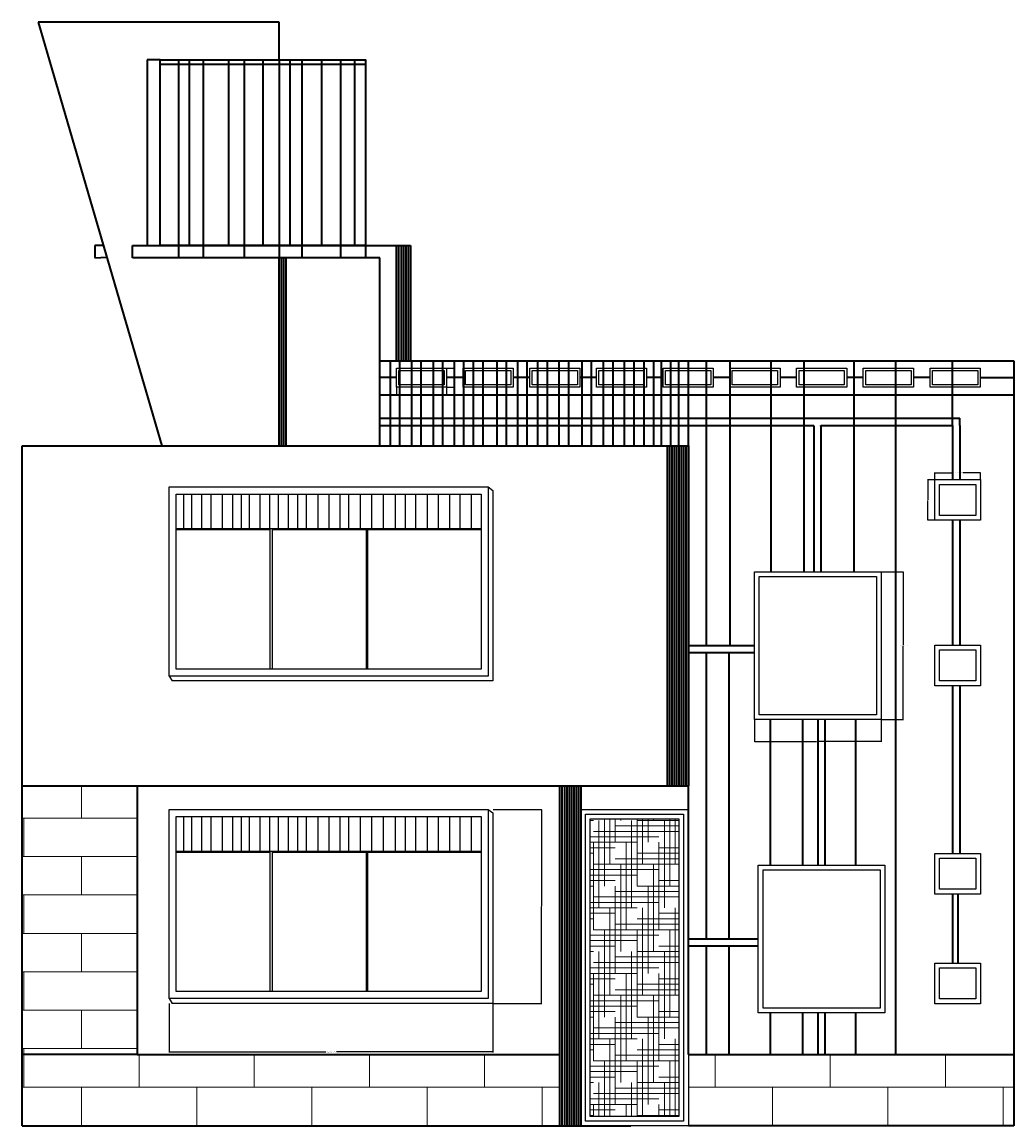
# Model space of a CAD drawing. Units: inches. Extents: x 72 to 493, y 65 to 532.
import ezdxf

# ---------------------------------------------------------------- set-up
doc = ezdxf.new("R2010")
doc.units = ezdxf.units.IN
doc.header["$MEASUREMENT"] = 0
for name, color, linetype, lineweight in [('A-ANNO-DIMS', 2, 'Continuous', 18), ('A-DOOR', 3, 'Continuous', 25), ('A-DOOR-PATT', 8, 'Continuous', 13), ('A-ELEV', 7, 'Continuous', 35), ('A-GLAZ', 4, 'Continuous', 25), ('A-WALL-PATT', 8, 'Continuous', 13)]:
    doc.layers.add(name, color=color, linetype=linetype, lineweight=lineweight)
doc.styles.get("Standard").update_dxf_attribs({"font": 'arial.ttf'})
doc.dimstyles.get("Standard").update_dxf_attribs({"dimtxt": 0.18, "dimasz": 0.18, "dimexe": 0.18, "dimexo": 0.0625, "dimgap": 0.09, "dimtad": 0, "dimtih": 1, "dimtoh": 1, "dimdec": 4, "dimzin": 0, "dimdsep": 46, "dimtxsty": 'Standard', "dimcen": 0.09, "dimadec": 0, "dimazin": 0, "dimtfac": 1, "dimtdec": 4, "dimtofl": 0, "dimtmove": 0, "dimatfit": 3, "dimfxl": 1, "dimtolj": 1, "dimtzin": 0, "dimarcsym": 0})

# ---------------------------------------------------------------- blocks, each defined once
blk = doc.blocks.new('WIN-SLIDING-3P')
for p, q in [((135.19, 82.11), (137.19, 80.63)), ((6.15, 79.11), (6.15, 64.5)), ((9.47, 79.11), (9.47, 64.5)), ((13.66, 79.11), (13.66, 64.5)), ((17.62, 79.11), (17.62, 64.5)), ((22.45, 79.11), (22.45, 64.5)), ((26.79, 79.11), (26.79, 64.5)), ((30.5, 79.11), (30.5, 64.5)), ((33.96, 79.11), (33.96, 64.5)), ((38.45, 79.11), (38.45, 64.5)), ((42.5, 79.11), (42.5, 64.5)), ((46.21, 79.11), (46.21, 64.5)), ((50.45, 79.11), (50.45, 64.5)), ((54.35, 79.11), (54.35, 64.5)), ((58.03, 79.11), (58.03, 64.5)), ((62.95, 79.11), (62.95, 64.5)), ((67.59, 79.11), (67.59, 64.5)), ((72.27, 79.11), (72.27, 64.5)), ((75.98, 79.11), (75.98, 64.5)), ((80.86, 79.11), (80.86, 64.5)), ((85.7, 79.11), (85.7, 64.5)), ((90.63, 79.11), (90.63, 64.5)), ((95.8, 79.11), (95.8, 64.5)), ((100.04, 79.11), (100.04, 64.5)), ((104.4, 79.11), (104.4, 64.5)), ((109.37, 79.11), (109.37, 64.5)), ((113.96, 79.11), (113.96, 64.5)), ((118.79, 79.11), (118.79, 64.5)), ((123.13, 79.11), (123.13, 64.5)), ((128.01, 79.11), (128.01, 64.5)), ((3, 64.5), (132.19, 64.5)), ((0, 2), (1.28, 0))]:
    blk.add_line(p, q)
for points in [[(0, 82.11), (135.19, 82.11), (135.19, 2), (0, 2)], [(3, 79.11), (132.19, 79.11), (132.19, 5), (3, 5)], [(3, 64.05), (42.69, 64.05), (42.69, 5), (3, 5)], [(43.75, 64.05), (83.44, 64.05), (83.44, 5), (43.75, 5)], [(84.24, 64.05), (132.19, 64.05), (132.19, 5), (84.24, 5)]]:
    blk.add_lwpolyline(points, close=True)
blk.add_lwpolyline([(137.19, 80.63), (137.19, 0), (1.28, 0)])
blk = doc.blocks.new('WIN-CLERESTORY')
for points in [[(0, 8.05), (21.2, 8.05), (21.2, 0), (0, 0)], [(1, 7.05), (20.2, 7.05), (20.2, 1), (1, 1)]]:
    blk.add_lwpolyline(points, close=True)
blk = doc.blocks.new('WIN-SQ-SMALL')
for points in [[(0, 17.16), (19.41, 17.16), (19.41, 0), (0, 0)], [(2, 15.16), (17.41, 15.16), (17.41, 2), (2, 2)]]:
    blk.add_lwpolyline(points, close=True)
blk = doc.blocks.new('WIN-SQ-LARGE')
for points in [[(0, 62.56), (53.66, 62.56), (53.66, 0), (0, 0)], [(2, 60.56), (51.66, 60.56), (51.66, 2), (2, 2)]]:
    blk.add_lwpolyline(points, close=True)
blk = doc.blocks.new('*D5')
at = {"layer": 'A-ANNO-DIMS', "color": 0, "lineweight": -2, "transparency": 16777216}
for p, q in [((231.1, 377.71), (231.1, 374.41)), ((231.28, 374.59), (239.7, 374.59)), ((252.13, 374.59), (243.7, 374.59)), ((252.31, 377.71), (252.31, 374.41))]:
    blk.add_line(p, q, dxfattribs=at)
at = {"layer": 'A-ANNO-DIMS', "color": 0, "transparency": 16777216}
for points in [[(231.28, 374.62), (231.28, 374.56), (231.1, 374.59)], [(252.13, 374.62), (252.13, 374.56), (252.31, 374.59)]]:
    blk.add_solid(points, dxfattribs=at)
at = {"layer": 'Defpoints', "color": 0, "transparency": 16777216}
for p in [(231.1, 377.77), (252.31, 377.77), (252.31, 374.59)]:
    blk.add_point(p, dxfattribs=at)
at = {"layer": 'A-ANNO-DIMS', "color": 0, "transparency": 16777216, "insert": (241.7, 374.59), "char_height": 0.18, "attachment_point": 5}
blk.add_mtext('\\A1;CLERESTORY WINDOW 21 TYP.', dxfattribs=at)
blk = doc.blocks.new('*D6')
at = {"layer": 'A-ANNO-DIMS', "color": 0, "lineweight": -2, "transparency": 16777216}
for p, q in [((252.37, 385.83), (255.67, 385.83)), ((255.49, 385.65), (255.49, 381.98)), ((255.49, 377.95), (255.49, 381.62)), ((252.37, 377.77), (255.67, 377.77))]:
    blk.add_line(p, q, dxfattribs=at)
at = {"layer": 'A-ANNO-DIMS', "color": 0, "transparency": 16777216}
for points in [[(255.46, 385.65), (255.52, 385.65), (255.49, 385.83)], [(255.46, 377.95), (255.52, 377.95), (255.49, 377.77)]]:
    blk.add_solid(points, dxfattribs=at)
at = {"layer": 'Defpoints', "color": 0, "transparency": 16777216}
for p in [(252.31, 385.83), (255.49, 385.83), (252.31, 377.77)]:
    blk.add_point(p, dxfattribs=at)
at = {"layer": 'A-ANNO-DIMS', "color": 0, "transparency": 16777216, "insert": (255.49, 381.8), "char_height": 0.18, "attachment_point": 5}
blk.add_mtext('\\A1;8 TYP.', dxfattribs=at)
blk = doc.blocks.new('*D7')
at = {"layer": 'A-ANNO-DIMS', "color": 0, "lineweight": -2, "transparency": 16777216}
for p, q in [((459.13, 338.66), (459.13, 341.69)), ((459.31, 341.51), (466.71, 341.51)), ((478.36, 341.51), (470.96, 341.51)), ((478.54, 338.66), (478.54, 341.69))]:
    blk.add_line(p, q, dxfattribs=at)
at = {"layer": 'A-ANNO-DIMS', "color": 0, "transparency": 16777216}
for points in [[(459.31, 341.54), (459.31, 341.48), (459.13, 341.51)], [(478.36, 341.54), (478.36, 341.48), (478.54, 341.51)]]:
    blk.add_solid(points, dxfattribs=at)
at = {"layer": 'Defpoints', "color": 0, "transparency": 16777216}
for p in [(478.54, 341.51), (459.13, 338.59), (478.54, 338.59)]:
    blk.add_point(p, dxfattribs=at)
at = {"layer": 'A-ANNO-DIMS', "color": 0, "transparency": 16777216, "insert": (468.84, 341.51), "char_height": 0.18, "attachment_point": 5}
blk.add_mtext('\\A1;SMALL SQUARE WINDOW 19 TYP.', dxfattribs=at)
blk = doc.blocks.new('*D8')
at = {"layer": 'A-ANNO-DIMS', "color": 0, "lineweight": -2, "transparency": 16777216}
for p, q in [((459.07, 338.59), (456.04, 338.59)), ((456.22, 338.41), (456.22, 330.2)), ((456.22, 321.62), (456.22, 329.83)), ((459.07, 321.44), (456.04, 321.44))]:
    blk.add_line(p, q, dxfattribs=at)
at = {"layer": 'A-ANNO-DIMS', "color": 0, "transparency": 16777216}
for points in [[(456.19, 338.41), (456.25, 338.41), (456.22, 338.59)], [(456.19, 321.62), (456.25, 321.62), (456.22, 321.44)]]:
    blk.add_solid(points, dxfattribs=at)
at = {"layer": 'Defpoints', "color": 0, "transparency": 16777216}
for p in [(456.22, 338.59), (459.13, 338.59), (459.13, 321.44)]:
    blk.add_point(p, dxfattribs=at)
at = {"layer": 'A-ANNO-DIMS', "color": 0, "transparency": 16777216, "insert": (456.22, 330.02), "char_height": 0.18, "attachment_point": 5}
blk.add_mtext('\\A1;17 TYP.', dxfattribs=at)
blk = doc.blocks.new('*D9')
at = {"layer": 'A-ANNO-DIMS', "color": 0, "lineweight": -2, "transparency": 16777216}
for p, q in [((134.75, 116.73), (134.75, 96.04)), ((271.94, 116.73), (271.94, 96.04)), ((134.93, 96.22), (201.07, 96.22)), ((271.76, 96.22), (205.63, 96.22))]:
    blk.add_line(p, q, dxfattribs=at)
at = {"layer": 'A-ANNO-DIMS', "color": 0, "transparency": 16777216}
for points in [[(134.93, 96.25), (134.93, 96.19), (134.75, 96.22)], [(271.76, 96.25), (271.76, 96.19), (271.94, 96.22)]]:
    blk.add_solid(points, dxfattribs=at)
at = {"layer": 'Defpoints', "color": 0, "transparency": 16777216}
for p in [(134.75, 116.8), (271.94, 116.8), (271.94, 96.22)]:
    blk.add_point(p, dxfattribs=at)
at = {"layer": 'A-ANNO-DIMS', "color": 0, "transparency": 16777216, "insert": (203.35, 96.22), "char_height": 0.18, "attachment_point": 5}
blk.add_mtext('\\A1;3-PANEL SLIDING WINDOW 137 TYP.', dxfattribs=at)
blk = doc.blocks.new('*D10')
at = {"layer": 'A-ANNO-DIMS', "color": 0, "lineweight": -2, "transparency": 16777216}
for p, q in [((272, 198.91), (292.7, 198.91)), ((292.52, 198.73), (292.52, 158.03)), ((292.52, 116.98), (292.52, 157.67)), ((272, 116.8), (292.7, 116.8))]:
    blk.add_line(p, q, dxfattribs=at)
at = {"layer": 'A-ANNO-DIMS', "color": 0, "transparency": 16777216}
for points in [[(292.49, 198.73), (292.55, 198.73), (292.52, 198.91)], [(292.49, 116.98), (292.55, 116.98), (292.52, 116.8)]]:
    blk.add_solid(points, dxfattribs=at)
at = {"layer": 'Defpoints', "color": 0, "transparency": 16777216}
for p in [(271.94, 198.91), (292.52, 198.91), (271.94, 116.8)]:
    blk.add_point(p, dxfattribs=at)
at = {"layer": 'A-ANNO-DIMS', "color": 0, "transparency": 16777216, "insert": (292.52, 157.85), "char_height": 0.18, "attachment_point": 5}
blk.add_mtext('\\A1;82 TYP.', dxfattribs=at)
blk = doc.blocks.new('*D11')
at = {"layer": 'A-ANNO-DIMS', "color": 0, "lineweight": -2, "transparency": 16777216}
for p, q in [((436.42, 299.62), (445.92, 299.62)), ((445.74, 299.44), (445.74, 268.53)), ((445.74, 237.24), (445.74, 268.15)), ((436.42, 237.06), (445.92, 237.06))]:
    blk.add_line(p, q, dxfattribs=at)
at = {"layer": 'A-ANNO-DIMS', "color": 0, "transparency": 16777216}
for points in [[(445.71, 299.44), (445.77, 299.44), (445.74, 299.62)], [(445.71, 237.24), (445.77, 237.24), (445.74, 237.06)]]:
    blk.add_solid(points, dxfattribs=at)
at = {"layer": 'Defpoints', "color": 0, "transparency": 16777216}
for p in [(436.35, 299.62), (445.74, 299.62), (436.35, 237.06)]:
    blk.add_point(p, dxfattribs=at)
at = {"layer": 'A-ANNO-DIMS', "color": 0, "transparency": 16777216, "insert": (445.74, 268.34), "char_height": 0.18, "attachment_point": 5}
blk.add_mtext('\\A1;LARGE SQUARE WINDOW 63 TYP.', dxfattribs=at)
blk = doc.blocks.new('*D12')
at = {"layer": 'A-ANNO-DIMS', "color": 0, "lineweight": -2, "transparency": 16777216}
for p, q in [((382.7, 237), (382.7, 227.5)), ((436.35, 237), (436.35, 227.5)), ((382.88, 227.68), (409, 227.68)), ((436.17, 227.68), (410.05, 227.68))]:
    blk.add_line(p, q, dxfattribs=at)
at = {"layer": 'A-ANNO-DIMS', "color": 0, "transparency": 16777216}
for points in [[(382.88, 227.71), (382.88, 227.65), (382.7, 227.68)], [(436.17, 227.71), (436.17, 227.65), (436.35, 227.68)]]:
    blk.add_solid(points, dxfattribs=at)
at = {"layer": 'Defpoints', "color": 0, "transparency": 16777216}
for p in [(382.7, 237.06), (436.35, 237.06), (436.35, 227.68)]:
    blk.add_point(p, dxfattribs=at)
at = {"layer": 'A-ANNO-DIMS', "color": 0, "transparency": 16777216, "insert": (409.53, 227.68), "char_height": 0.18, "attachment_point": 5}
blk.add_mtext('\\A1;54 TYP.', dxfattribs=at)

msp = doc.modelspace()

# ---------------------------------------------------------------- hatches: boundary and pattern name
at = {"layer": 'A-DOOR-PATT'}
h = msp.add_hatch(dxfattribs=at)
h.set_pattern_fill('HOUND', color=256, scale=37)
h.paths.add_polyline_path([(350.71, 194.91), (313.18, 194.91), (313.18, 68.9), (350.71, 68.9)])
at = {"layer": 'A-WALL-PATT'}
h = msp.add_hatch(dxfattribs=at)
h.set_pattern_fill('AR-BRSTD', color=256, scale=6.1)
h.paths.add_polyline_path([(121.24, 208.9), (72.44, 208.9), (72.44, 95.18), (121.24, 95.18), (121.24, 102.65)])
h.paths.add_polyline_path([(300.18, 95.18), (121.24, 95.18), (72.44, 95.18), (72.44, 64.9), (300.18, 64.9)])
h = msp.add_hatch(dxfattribs=at)
h.set_pattern_fill('AR-BRSTD', color=256, scale=6.1)
h.paths.add_polyline_path([(492.65, 95.18), (354.71, 95.18), (354.71, 64.9), (492.65, 64.9)])

# ---------------------------------------------------------------- linework, layer by layer
at = {"layer": 'A-DOOR'}
for points in [[(309.18, 198.91), (354.71, 198.91), (354.71, 64.9), (309.18, 64.9)], [(311.18, 196.91), (352.71, 196.91), (352.71, 66.9), (311.18, 66.9)], [(313.18, 194.91), (350.71, 194.91), (350.71, 68.9), (313.18, 68.9)]]:
    msp.add_lwpolyline(points, close=True, dxfattribs=at)
at = {"layer": 'A-ELEV'}
for p, q in [((181.34, 532.39), (79.24, 532.39)), ((79.24, 532.39), (131.59, 352.9)), ((181.34, 516.41), (181.34, 532.39)), ((130.98, 516.41), (125.38, 516.41)), ((125.38, 516.41), (125.38, 437.74)), ((130.98, 514.51), (218, 514.51)), ((138.73, 516.41), (138.73, 437.74)), ((143.2, 516.41), (143.2, 437.74)), ((149.17, 516.41), (149.17, 437.74)), ((159.92, 516.41), (159.92, 437.74)), ((166.48, 516.41), (166.48, 437.74)), ((174.49, 516.41), (174.49, 437.74)), ((181.34, 516.41), (181.34, 437.74)), ((185.88, 516.41), (185.88, 437.74)), ((190.95, 516.41), (190.95, 437.74)), ((199.31, 516.41), (199.31, 437.74)), ((199.31, 516.41), (199.31, 437.74)), ((207.37, 516.41), (207.37, 437.74)), ((213.34, 516.41), (213.34, 437.74)), ((106.84, 437.74), (103.24, 437.74)), ((103.24, 437.74), (103.24, 432.6)), ((119.28, 432.6), (119.28, 437.74)), ((119.28, 437.74), (230.98, 437.74)), ((138.73, 437.74), (138.73, 432.6)), ((149.17, 437.74), (149.17, 432.6)), ((166.48, 437.74), (166.48, 432.6)), ((181.34, 437.74), (181.34, 432.6)), ((190.95, 437.74), (190.95, 432.6)), ((207.37, 437.74), (207.37, 432.6)), ((218, 437.74), (218, 432.6)), ((230.98, 437.74), (230.98, 388.9)), ((230.98, 437.74), (236.98, 437.74)), ((231.98, 437.74), (231.98, 388.9)), ((232.98, 437.74), (232.98, 388.9)), ((233.98, 437.74), (233.98, 388.9)), ((234.98, 437.74), (234.98, 388.9)), ((235.98, 437.74), (235.98, 388.9)), ((236.98, 437.74), (236.98, 388.9)), ((103.24, 432.6), (108.29, 432.8)), ((224.06, 432.6), (119.28, 432.6)), ((181.34, 352.9), (181.34, 432.6)), ((182.34, 352.9), (182.34, 432.6)), ((183.34, 352.9), (183.34, 432.6)), ((184.34, 352.9), (184.34, 432.6)), ((224.06, 388.9), (224.06, 432.6)), ((224.06, 352.9), (224.06, 388.9)), ((224.06, 388.9), (492.65, 388.9)), ((228.5, 352.9), (228.5, 388.9)), ((232.5, 352.9), (232.5, 388.9)), ((237.54, 352.9), (237.54, 388.9)), ((241.54, 352.9), (241.54, 388.9)), ((246.69, 352.9), (246.69, 388.9)), ((250.69, 352.9), (250.69, 388.9)), ((255.58, 352.9), (255.58, 388.9)), ((259.58, 352.9), (259.58, 388.9)), ((263.75, 352.9), (263.75, 388.9)), ((267.75, 352.9), (267.75, 388.9)), ((273.73, 352.9), (273.73, 388.9)), ((277.73, 352.9), (277.73, 388.9)), ((282.49, 352.9), (282.49, 388.9)), ((286.49, 352.9), (286.49, 388.9)), ((290.99, 352.9), (290.99, 388.9)), ((294.99, 352.9), (294.99, 388.9)), ((300.02, 352.9), (300.02, 388.9)), ((304.02, 352.9), (304.02, 388.9)), ((309.7, 352.9), (309.7, 388.9)), ((313.7, 352.9), (313.7, 388.9)), ((318.81, 352.9), (318.81, 388.9)), ((322.81, 352.9), (322.81, 388.9)), ((327.72, 352.9), (327.72, 388.9)), ((331.72, 352.9), (331.72, 388.9)), ((336.05, 352.9), (336.05, 388.9)), ((340.05, 352.9), (340.05, 388.9)), ((343.28, 352.9), (343.28, 388.9)), ((347.28, 352.9), (347.28, 388.9)), ((350.71, 352.9), (350.71, 388.9)), ((354.71, 352.9), (354.71, 388.9)), ((362.31, 388.9), (362.31, 268.34)), ((372.27, 388.9), (372.27, 268.34)), ((389.6, 388.9), (389.6, 299.62)), ((403.62, 388.9), (403.62, 299.62)), ((424.97, 299.62), (424.97, 388.9)), ((442.47, 388.9), (442.47, 95.18)), ((466.69, 361.58), (466.69, 388.9)), ((492.65, 388.9), (492.65, 95.18)), ((231.1, 381.8), (224.06, 381.8)), ((259.35, 381.8), (252.31, 381.8)), ((287.6, 381.8), (280.55, 381.8)), ((315.85, 381.8), (308.8, 381.8)), ((344.09, 381.8), (337.05, 381.8)), ((372.34, 381.8), (365.3, 381.8)), ((400.59, 381.8), (393.55, 381.8)), ((428.84, 381.8), (421.79, 381.8)), ((457.09, 381.8), (450.04, 381.8)), ((478.29, 381.8), (492.65, 381.8)), ((224.06, 374.59), (492.65, 374.59)), ((224.06, 364.58), (469.69, 364.58)), ((224.06, 361.58), (403.1, 361.58)), ((403.1, 361.58), (406.1, 361.58)), ((406.1, 361.58), (407.88, 361.58)), ((407.88, 361.28), (407.88, 361.58)), ((407.88, 361.28), (407.88, 299.62)), ((410.88, 361.28), (410.88, 361.58)), ((410.88, 361.58), (466.69, 361.58)), ((410.88, 361.28), (410.88, 299.62)), ((466.69, 361.58), (466.69, 338.59)), ((469.69, 361.58), (469.69, 364.58)), ((469.69, 361.58), (469.69, 338.59)), ((72.44, 208.9), (72.44, 352.9)), ((72.44, 352.9), (354.71, 352.9)), ((345.71, 352.9), (345.71, 208.9)), ((346.71, 352.9), (346.71, 208.9)), ((347.71, 352.9), (347.71, 208.9)), ((348.71, 352.9), (348.71, 208.9)), ((349.71, 352.9), (349.71, 208.9)), ((350.71, 352.9), (350.71, 208.9)), ((351.71, 352.9), (351.71, 208.9)), ((352.71, 352.9), (352.71, 208.9)), ((353.71, 352.9), (353.71, 208.9)), ((354.71, 208.9), (354.71, 352.9)), ((354.71, 352.9), (354.71, 208.9)), ((466.69, 321.44), (466.69, 268.49)), ((469.69, 321.44), (469.69, 268.49)), ((354.71, 268.34), (382.7, 268.34)), ((354.71, 265.34), (382.7, 265.34)), ((362.31, 265.34), (362.31, 144.12)), ((371.89, 265.34), (371.89, 144.12)), ((466.69, 251.33), (466.69, 180.26)), ((469.69, 251.33), (469.69, 180.11)), ((389.36, 237.06), (389.36, 175.4)), ((403.01, 237.06), (403.01, 175.4)), ((409.53, 237.06), (409.53, 175.4)), ((412.53, 237.06), (412.53, 175.4)), ((425.56, 237.06), (425.56, 175.4)), ((72.44, 64.9), (72.44, 208.9)), ((72.44, 208.9), (329.76, 208.9)), ((121.24, 208.9), (121.24, 102.65)), ((300.18, 208.9), (300.18, 95.18)), ((301.18, 208.9), (301.18, 64.9)), ((302.18, 208.9), (302.18, 64.9)), ((303.18, 208.9), (303.18, 64.9)), ((304.18, 208.9), (304.18, 64.9)), ((305.18, 208.9), (305.18, 64.9)), ((306.18, 208.9), (306.18, 64.9)), ((307.18, 208.9), (307.18, 64.9)), ((308.18, 208.9), (308.18, 64.9)), ((309.18, 208.9), (309.18, 64.9)), ((329.76, 208.9), (354.71, 208.9)), ((354.71, 95.18), (354.71, 208.9)), ((466.69, 163.1), (466.69, 133.82)), ((468.84, 163.1), (468.84, 134.01)), ((354.71, 144.12), (384.34, 144.12)), ((354.71, 141.12), (384.34, 141.12)), ((362.31, 141.12), (362.31, 95.18)), ((371.89, 141.12), (371.89, 95.18)), ((389.36, 112.84), (389.36, 95.18)), ((403.01, 112.84), (403.01, 95.18)), ((409.53, 112.84), (409.53, 95.18)), ((412.53, 112.84), (412.53, 95.18)), ((425.56, 112.84), (425.56, 95.18)), ((121.24, 102.65), (121.24, 95.18)), ((121.24, 95.18), (72.44, 95.18)), ((121.24, 95.18), (300.18, 95.18)), ((300.18, 95.18), (300.18, 64.9)), ((354.71, 95.18), (492.65, 95.18)), ((492.65, 95.18), (492.65, 64.9)), ((72.44, 64.9), (330.31, 64.9)), ((492.65, 64.9), (354.71, 64.9))]:
    msp.add_line(p, q, dxfattribs=at)
msp.add_lwpolyline([(218, 437.74), (130.98, 437.74), (130.98, 516.41), (218, 516.41)], close=True, dxfattribs=at)

# ---------------------------------------------------------------- block references
at = {"layer": 'A-GLAZ'}
for name, p in [('WIN-CLERESTORY', (231.1, 377.77)), ('WIN-CLERESTORY', (259.35, 377.77)), ('WIN-CLERESTORY', (287.6, 377.77)), ('WIN-CLERESTORY', (315.85, 377.77)), ('WIN-CLERESTORY', (344.09, 377.77)), ('WIN-CLERESTORY', (372.34, 377.77)), ('WIN-CLERESTORY', (400.59, 377.77)), ('WIN-CLERESTORY', (428.84, 377.77)), ('WIN-CLERESTORY', (457.09, 377.77)), ('WIN-SQ-SMALL', (459.13, 321.44)), ('WIN-SLIDING-3P', (134.75, 253.4)), ('WIN-SQ-LARGE', (382.7, 237.06)), ('WIN-SQ-SMALL', (459.13, 251.33)), ('WIN-SLIDING-3P', (134.75, 116.8)), ('WIN-SQ-SMALL', (459.13, 163.1)), ('WIN-SQ-LARGE', (384.34, 112.84)), ('WIN-SQ-SMALL', (459.13, 116.66))]:
    msp.add_blockref(name, p, dxfattribs=at)

# ---------------------------------------------------------------- dimensions: what is measured, and where the dimension line sits
at = {"layer": 'A-ANNO-DIMS'}
for base, p1, p2, text, picture, middle in [((255.49, 385.83), (252.31, 377.77), (252.31, 385.83), '<> TYP.', '*D6', (255.49, 381.8)), ((456.22, 338.59), (459.13, 321.44), (459.13, 338.59), '<> TYP.', '*D8', (456.22, 330.02)), ((445.74, 299.62), (436.35, 237.06), (436.35, 299.62), 'LARGE SQUARE WINDOW <> TYP.', '*D11', (445.74, 268.34)), ((292.52, 198.91), (271.94, 116.8), (271.94, 198.91), '<> TYP.', '*D10', (292.52, 157.85))]:
    dim = msp.add_linear_dim(base=base, p1=p1, p2=p2, angle=90, text=text, dimstyle='Standard', override={"dimdec": 0, "dimlfac": 1, "dimrnd": 0, "dimzin": 0, "dimdsep": 46, "dimlunit": 2}, dxfattribs=at)
    dim.commit()
    dim.dimension.update_dxf_attribs({"geometry": picture, "text_midpoint": middle})
for base, p1, p2, text, picture, middle in [((252.31, 374.59), (231.1, 377.77), (252.31, 377.77), 'CLERESTORY WINDOW <> TYP.', '*D5', (241.7, 374.59)), ((478.54, 341.51), (459.13, 338.59), (478.54, 338.59), 'SMALL SQUARE WINDOW <> TYP.', '*D7', (468.84, 341.51)), ((436.35, 227.68), (382.7, 237.06), (436.35, 237.06), '<> TYP.', '*D12', (409.53, 227.68)), ((271.94, 96.22), (134.75, 116.8), (271.94, 116.8), '3-PANEL SLIDING WINDOW <> TYP.', '*D9', (203.35, 96.22))]:
    dim = msp.add_linear_dim(base=base, p1=p1, p2=p2, text=text, dimstyle='Standard', override={"dimdec": 0, "dimlfac": 1, "dimrnd": 0, "dimzin": 0, "dimdsep": 46, "dimlunit": 2}, dxfattribs=at)
    dim.commit()
    dim.dimension.update_dxf_attribs({"geometry": picture, "text_midpoint": middle})

doc.saveas('drawing.dxf')
